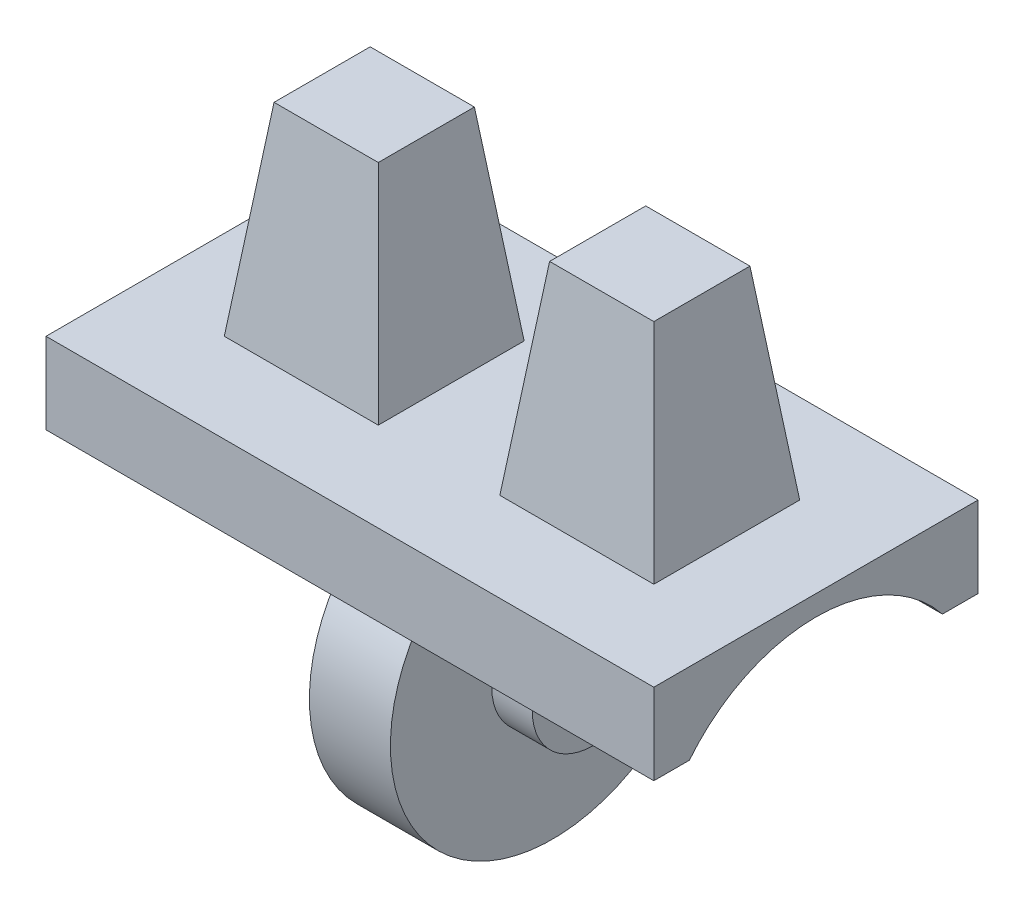
SolidWorks part; units mm, degrees
material "Plain Carbon Steel"
ref_plane "Front Plane" through (0, 0, 0) normal (0, 0, 1) x (1, 0, 0)
ref_plane "Top Plane" through (0, 0, 0) normal (0, 1, 0) x (1, 0, 0)
ref_plane "Right Plane" through (0, 0, 0) normal (1, 0, 0) x (0, 0, -1)
sketch "Base Plate Sketch" plane through (0, 0, 0) normal (0, 1, 0) x (1, 0, 0)
  line L1 (0, 0) -> (15, 0)
  line L2 (0, 0) -> (0, 8)
  line L3 (0, 8) -> (15, 8)
  line L4 (15, 0) -> (15, 8)
  dimension "D1" = 8
  dimension "D2" = 15
extrude "Base Plate 15x8x2" add sketch "Base Plate Sketch" along normal blind 2 separate body
sketch "Hip Blocks Sketch" plane through (0, 2, 0) normal (0, 1, 0) x (1, 0, 0)
  line L0 (7.5, 8) -> (7.5, 0) construction
  line L1 (15, 8) -> (0, 8) construction
  line L2 (0, 0) -> (15, 0) construction
  line L3 (0, 8) -> (0, 0) construction
  line L4 (2.2, 5.8) -> (6, 5.8)
  line L5 (2.2, 5.8) -> (2.2, 2.2)
  line L6 (2.2, 2.2) -> (6, 2.2)
  line L7 (6, 5.8) -> (6, 2.2)
  line L8 (12.8, 5.8) -> (12.8, 2.2)
  line L9 (12.8, 5.8) -> (9, 5.8)
  line L10 (9, 5.8) -> (9, 2.2)
  line L11 (12.8, 2.2) -> (9, 2.2)
  dimension "D1" = 1.5
  dimension "D2" = 2.2
  dimension "D3" = 2.2
  dimension "D4" = 2.2
extrude "Hip Blocks Drafted 5mm" add sketch "Hip Blocks Sketch" along normal blind 5 draft 7
sketch "Underside Relief Sketch" plane through (15, 0, 0) normal (1, 0, 0) x (0, 0, -1)
  line L0 (4, 0) -> (4, -2.5) construction
  line L4 (0, 0) -> (8, 0)
  line L5 (8, 0) -> (8, 2)
  line L6 (8, 2) -> (0, 2)
  line L7 (0, 2) -> (0, 0)
  line L8 (0, 0) -> (8, 0)
  line L9 (8, 0) -> (8, 2)
  line L10 (8, 2) -> (0, 2)
  line L11 (0, 2) -> (0, 0)
  circle A0 centre (4, -2.5) radius 4
  dimension "D2" = 8
  dimension "D3" = 2.5
  dimension "D1" = 0
extrude "Underside Relief Cut" cut sketch "Underside Relief Sketch" against normal through all
ref_plane "Hip Disc Plane" through (7.5, 0, 0) normal (-1, 0, 0) x (0, 0, 1)
sketch "Hip Disc Sketch" plane through (7.5, 0, 0) normal (-1, 0, 0) x (0, 0, 1)
  circle A0 centre (-4, -2.5) radius 4
  dimension "D1" = 8
extrude "Hip Disc Ø8" add sketch "Hip Disc Sketch" along normal mid plane 2
sketch "Axle Pin A Sketch" plane through (8.5, 0, 0) normal (1, 0, 0) x (0, 0, -1)
  circle A0 centre (4, -2.5) radius 1.5
  dimension "D1" = 3
extrude "Axle Pin A Ø3" add sketch "Axle Pin A Sketch" along normal mid plane 2
sketch "Axle Pin B Sketch" plane through (6.5, 0, 0) normal (-1, 0, 0) x (0, 0, 1)
  circle A0 centre (-4, -2.5) radius 1.5
  dimension "D1" = 3
extrude "Axle Pin B Ø3" add sketch "Axle Pin B Sketch" along normal mid plane 2
